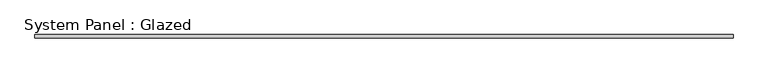
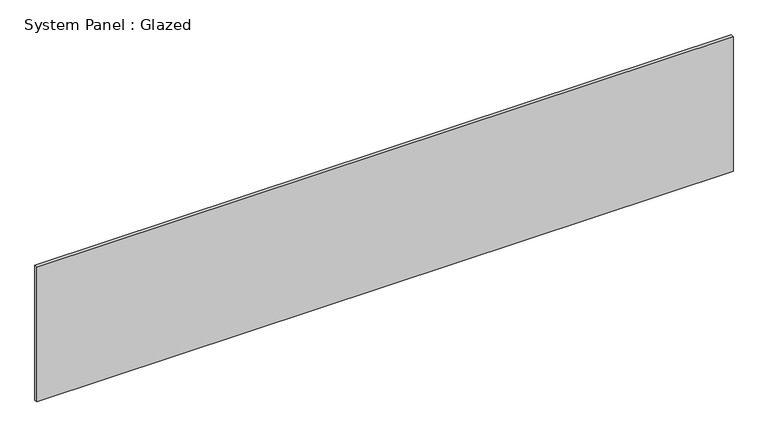
"""IFC4 building model written with IfcOpenShell, lengths in millimetres: plate geometry, System Panel : Glazed."""

from ifc_helpers import new_model, si_unit, origin, origin_with_axes, place, context, project, spatial, polyline, outline, extrude, source, transform, mapped, element, save


def system_panel_glazed_1356a548(model_context):
    return source(origin(), model_context, "Body", "SweptSolid", [
        extrude(outline(polyline([(2647.95, 19.05), (-2647.95, 19.05), (-2647.95, 44.45), (2647.95, 44.45), (2647.95, 19.05)])), origin_with_axes(), (0.0, 0.0, 1.0), 1082.2631063),
    ])


if __name__ == "__main__":
    model = new_model("IFC4")
    model_context = context("Model", 3, world=origin())
    ifc_project = project(units=[si_unit("LENGTHUNIT", "METRE", prefix="MILLI")], contexts=[model_context])
    site = spatial("IfcSite", under=ifc_project)
    building = spatial("IfcBuilding", under=site)
    placement = place(None, origin())
    system_panel_glazed_shape = system_panel_glazed_1356a548(model_context)
    element("IfcPlate", 1, ObjectType="System Panel : Glazed", at=placement, inside=building, context=model_context, shape_type="MappedRepresentation", body=[
        mapped(system_panel_glazed_shape, transform((0.0, 0.0, 0.0), x_axis=(1.0, 0.0, 0.0), y_axis=(0.0, 1.0, 0.0), z_axis=(0.0, 0.0, 1.0))),
    ])
    save(model, "model.ifc")

# Revit data of these elements
# Type "System Panel : Glazed"
#   Construction Type Id = "GSP4R"
#   Analytic Construction = "1/8 in Pilkington single glazing"
#   Visual Light Transmittance = 0.9
#   Solar Heat Gain Coefficient = 0.86
#   Heat Transfer Coefficient (U) = 1.18115 BTU/(h·ft²·°F)
#   Define Thermal Properties by = 1
# Element 1 (IfcPlate, "System Panel : Glazed")
#   Materials on its faces: "Glass"
# Materials
#   "Glass": class "Glass", colour RGB 0 128 192, transparency 0.75, Description = "Soda Lime Glass", Cost = 0
